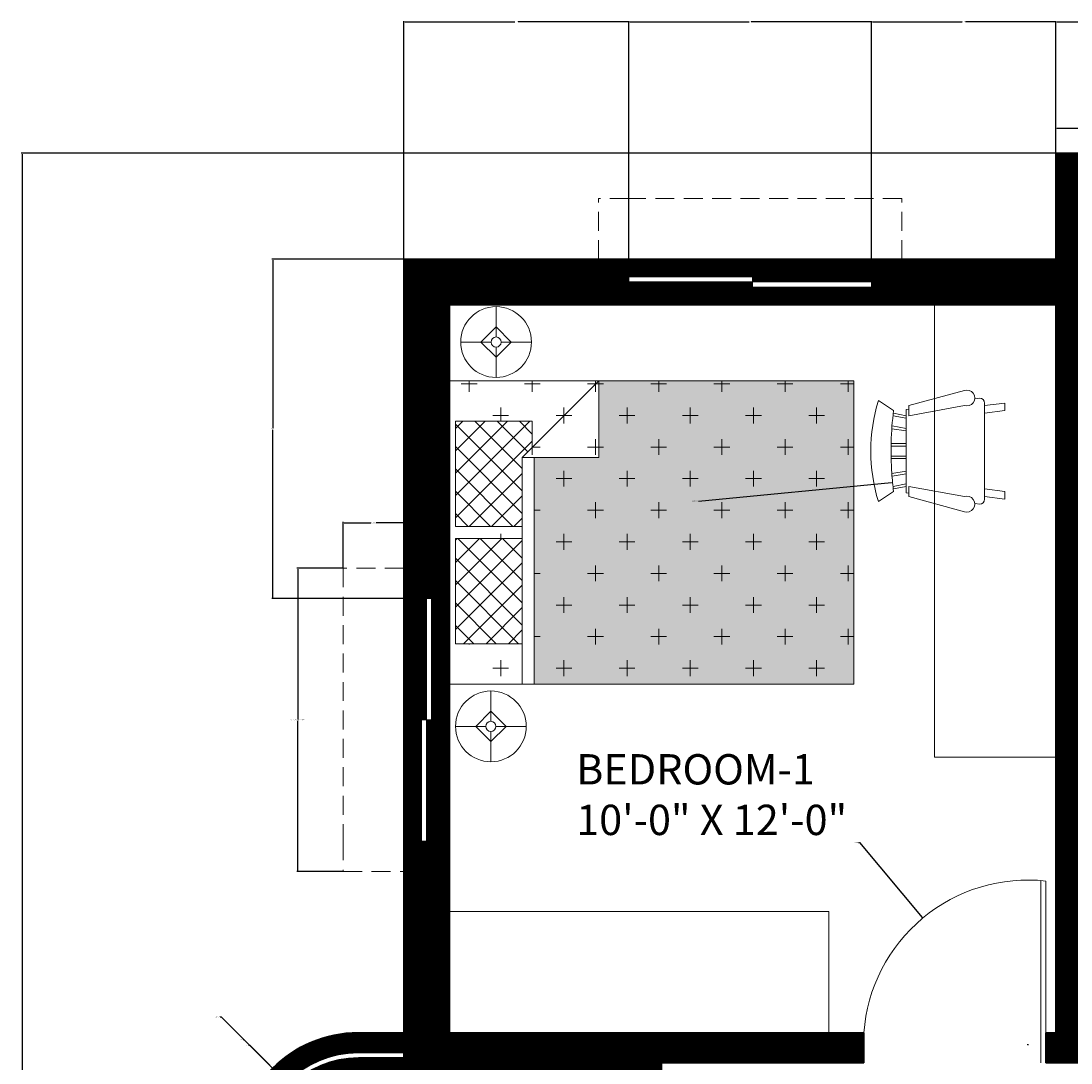
# Model space of a CAD drawing. Units: inches. Extents: x 557 to 1007, y 390 to 953.
# Tile 8 of 10: x 557 to 764, y 747 to 953. Entities that reach past the tile are written whole.
import ezdxf

# ---------------------------------------------------------------- set-up
doc = ezdxf.new("R2010")
doc.units = ezdxf.units.IN
doc.header["$LTSCALE"] = 5
doc.header["$MEASUREMENT"] = 0
doc.linetypes.add('HIDDEN', pattern=[0.375, 0.25, -0.125])
for name, color, linetype, lineweight in [('A-ANNO-DIMS', 2, 'Continuous', 18), ('A-AREA-IDEN', 7, 'Continuous', 18), ('A-DOOR', 3, 'Continuous', 18), ('A-FLOR-CASE', 8, 'Continuous', 18), ('A-FLOR-RAIL', 7, 'Continuous', 25), ('A-FURN', 8, 'Continuous', 18), ('A-FURN-PATT', 9, 'Continuous', 9), ('A-GLAZ', 4, 'Continuous', 18), ('A-GLAZ-OVHD', 8, 'HIDDEN', 13), ('A-WALL', 7, 'Continuous', 35), ('E-LITE', 2, 'Continuous', 13)]:
    doc.layers.add(name, color=color, linetype=linetype, lineweight=lineweight)
doc.layers.add('A-GLAZ-PATT', color=141, linetype='Continuous', lineweight=9, true_color=0xadddf7)
doc.layers.add('A-WALL-PATT', color=251, linetype='Continuous', lineweight=9, true_color=0x636466)
doc.styles.get("Standard").update_dxf_attribs({"font": 'arial.ttf'})
doc.dimstyles.get("Standard").update_dxf_attribs({"dimtxt": 0.18, "dimasz": 0.18, "dimexe": 0.18, "dimexo": 0.0625, "dimgap": 0.09, "dimtad": 0, "dimtih": 1, "dimtoh": 1, "dimdec": 4, "dimzin": 0, "dimdsep": 46, "dimtxsty": 'Standard', "dimcen": 0.09, "dimadec": 0, "dimazin": 0, "dimtfac": 1, "dimtdec": 4, "dimtofl": 0, "dimtmove": 0, "dimatfit": 3, "dimfxl": 1, "dimtolj": 1, "dimtzin": 0, "dimarcsym": 0})

# ---------------------------------------------------------------- blocks, each defined once
blk = doc.blocks.new('Chair - Rocking')
for p, q in [((-8, -4.5), (-10, -1.5)), ((8, -4.5), (10, -1.5)), ((-1.5, -4.05012), (-1.5, -7)), ((-1, -7), (-1, -4.05012)), ((1, -7), (1, -4.04655)), ((1.5, -4.05012), (1.5, -7)), ((-7.5, -4.5), (-7, -7)), ((-6.5, -7), (-7.02225, -4.43)), ((-4.5, -7), (-4.96674, -4.19951)), ((-4, -7), (-4.40532, -4.16272)), ((4, -7), (4.40187, -4.18694)), ((4.5, -7), (4.96761, -4.19437)), ((6.5, -7), (7, -4.4057)), ((7.5, -4.5), (7, -7)), ((-9, -7.5), (-12, -18.49999)), ((-7, -7.5), (-9, -7.5)), ((-9, -18.49999), (-7, -7.5)), ((-8.23428, -6.99939), (-8.3093, -7.47958)), ((-8.23041, -7), (8.23915, -7)), ((7, -7.5), (9, -7.5)), ((9, -18.49999), (7, -7.5)), ((8.31071, -7.48854), (8.23449, -7.00073)), ((9, -7.5), (12, -18.49999)), ((-10.36644, -20.64523), (-10.5, -21.49999)), ((10.5, -21.49999), (10.3575, -20.58798)), ((-9, -22.49999), (-9.5, -26.49999)), ((0, -22.49999), (-9.5, -22.49999)), ((-8, -26.49999), (-7.5, -22.49999)), ((0, -22.49999), (9.5, -22.49999)), ((8, -26.49999), (7.5, -22.49999)), ((9, -22.49999), (9.5, -26.49999)), ((-9.5, -26.49999), (-8, -26.49999)), ((9.5, -26.49999), (8, -26.49999))]:
    blk.add_line(p, q)
for centre, radius, start, end in [((0, -34.08333), 34.08333, 72.93847, 107.0615), ((0, -68.25004), 64.25, 93.92211, 97.15267), ((0, -68.25004), 64.25, 82.84733, 93.92211), ((-10.5, -18.99999), 1.58114, 161.5651, 18.43495), ((10.5, -18.99999), 1.58114, 161.5651, 18.43495), ((-9.5, -21.49999), 1, 180, 270), ((9.5, -21.49999), 1, 270, 0)]:
    blk.add_arc(centre, radius, start, end)
blk = doc.blocks.new('Lamp - Table')
for p, q in [((0, 7), (0, 1)), ((0, 3), (-3, 0)), ((3, 0), (0, 3)), ((-1, 0), (-7, 0)), ((-3, 0), (0, -3)), ((0, -3), (3, 0)), ((1, 0), (7, 0)), ((0, -1), (0, -7))]:
    blk.add_line(p, q)
for radius in [7, 1]:
    blk.add_circle((0, 0), radius)
blk = doc.blocks.new('BED-QUEEN-60x80-PLAN')
for p, q in [((0, 0), (0, 60)), ((0, 60), (80, 60)), ((29.6, 60), (14.4, 44.8)), ((29.6, 44.8), (29.6, 60)), ((80, 60), (80, 0)), ((1.2, 52), (16.4, 52)), ((1.2, 31.2), (1.2, 52)), ((16.4, 52), (16.4, 46.8)), ((14.4, 0), (14.4, 44.8)), ((14.4, 44.8), (29.6, 44.8)), ((16.8, 44.8), (16.8, 0)), ((14.4, 31.2), (1.2, 31.2)), ((1.2, 28.8), (14.4, 28.8)), ((1.2, 8), (1.2, 28.8)), ((14.4, 8), (1.2, 8)), ((80, 0), (0, 0))]:
    blk.add_line(p, q)
blk = doc.blocks.new('WIN-48-SLIDING')
for p, q in [((0, 9), (0, 0)), ((48, 9), (48, 0)), ((24, 5.5), (0, 5.5)), ((48, 4.5), (0, 4.5)), ((24, 5.5), (24, 3.5)), ((48, 3.5), (24, 3.5))]:
    blk.add_line(p, q)
blk = doc.blocks.new('WINDOW-SHADE-60')
at = {"ltscale": 3}
for p, q in [((12, 60), (0, 60)), ((0, 60), (0, 6)), ((12, 54), (12, 60)), ((0, 6), (0, 0)), ((0, 0), (12, 0))]:
    blk.add_line(p, q, dxfattribs=at)
blk = doc.blocks.new('*D35')
at = {"layer": 'A-ANNO-DIMS', "color": 0, "lineweight": -2, "ltscale": 5, "transparency": 16777216}
for p, q in [((620.34, 844.77), (611.23, 844.77)), ((611.41, 844.59), (611.41, 814.95)), ((611.41, 784.95), (611.41, 814.59)), ((620.34, 784.77), (611.23, 784.77))]:
    blk.add_line(p, q, dxfattribs=at)
at = {"layer": 'A-ANNO-DIMS', "color": 0, "ltscale": 5, "transparency": 16777216}
for points in [[(611.38, 844.59), (611.44, 844.59), (611.41, 844.77)], [(611.38, 784.95), (611.44, 784.95), (611.41, 784.77)]]:
    blk.add_solid(points, dxfattribs=at)
at = {"layer": 'Defpoints', "color": 0, "ltscale": 5, "transparency": 16777216}
for p in [(611.41, 844.77), (620.41, 844.77), (620.41, 784.77)]:
    blk.add_point(p, dxfattribs=at)
at = {"layer": 'A-ANNO-DIMS', "color": 0, "ltscale": 5, "transparency": 16777216, "insert": (611.41, 814.77), "char_height": 0.18, "attachment_point": 5}
blk.add_mtext('\\A1;WINDOW SHADE 60 TYP.', dxfattribs=at)
blk = doc.blocks.new('*D36')
at = {"layer": 'A-ANNO-DIMS', "color": 0, "lineweight": -2, "ltscale": 5, "transparency": 16777216}
for p, q in [((620.41, 844.83), (620.41, 853.95)), ((620.59, 853.77), (625.89, 853.77)), ((632.23, 853.77), (626.92, 853.77)), ((632.41, 844.83), (632.41, 853.95))]:
    blk.add_line(p, q, dxfattribs=at)
at = {"layer": 'A-ANNO-DIMS', "color": 0, "ltscale": 5, "transparency": 16777216}
for points in [[(620.59, 853.8), (620.59, 853.74), (620.41, 853.77)], [(632.23, 853.8), (632.23, 853.74), (632.41, 853.77)]]:
    blk.add_solid(points, dxfattribs=at)
at = {"layer": 'Defpoints', "color": 0, "ltscale": 5, "transparency": 16777216}
for p in [(632.41, 853.77), (620.41, 844.77), (632.41, 844.77)]:
    blk.add_point(p, dxfattribs=at)
at = {"layer": 'A-ANNO-DIMS', "color": 0, "ltscale": 5, "transparency": 16777216, "insert": (626.41, 853.77), "char_height": 0.18, "attachment_point": 5}
blk.add_mtext('\\A1;12 TYP.', dxfattribs=at)
blk = doc.blocks.new('*D46')
at = {"layer": 'A-ANNO-DIMS', "color": 0, "lineweight": -2, "ltscale": 5, "transparency": 16777216}
for p, q in [((761.34, 926.9), (556.69, 926.9)), ((556.87, 926.72), (556.87, 671.59)), ((556.87, 416.08), (556.87, 671.22)), ((773.34, 415.9), (556.69, 415.9))]:
    blk.add_line(p, q, dxfattribs=at)
at = {"layer": 'A-ANNO-DIMS', "color": 0, "ltscale": 5, "transparency": 16777216}
for points in [[(556.84, 926.72), (556.9, 926.72), (556.87, 926.9)], [(556.84, 416.08), (556.9, 416.08), (556.87, 415.9)]]:
    blk.add_solid(points, dxfattribs=at)
at = {"layer": 'Defpoints', "color": 0, "ltscale": 5, "transparency": 16777216}
for p in [(556.87, 926.9), (761.41, 926.9), (773.41, 415.9)]:
    blk.add_point(p, dxfattribs=at)
at = {"layer": 'A-ANNO-DIMS', "color": 0, "ltscale": 5, "transparency": 16777216, "insert": (556.87, 671.4), "char_height": 0.18, "attachment_point": 5}
blk.add_mtext('\\A1;511', dxfattribs=at)
blk = doc.blocks.new('*D47')
at = {"layer": 'A-ANNO-DIMS', "color": 0, "lineweight": -2, "ltscale": 5, "transparency": 16777216}
for p, q in [((632.41, 905.97), (632.41, 953.03)), ((632.59, 952.85), (654.33, 952.85)), ((676.73, 952.85), (654.99, 952.85)), ((676.91, 905.97), (676.91, 953.03))]:
    blk.add_line(p, q, dxfattribs=at)
at = {"layer": 'A-ANNO-DIMS', "color": 0, "ltscale": 5, "transparency": 16777216}
for points in [[(632.59, 952.88), (632.59, 952.82), (632.41, 952.85)], [(676.73, 952.88), (676.73, 952.82), (676.91, 952.85)]]:
    blk.add_solid(points, dxfattribs=at)
at = {"layer": 'Defpoints', "color": 0, "ltscale": 5, "transparency": 16777216}
for p in [(676.91, 952.85), (632.41, 905.9), (676.91, 905.9)]:
    blk.add_point(p, dxfattribs=at)
at = {"layer": 'A-ANNO-DIMS', "color": 0, "ltscale": 5, "transparency": 16777216, "insert": (654.66, 952.85), "char_height": 0.18, "attachment_point": 5}
blk.add_mtext('\\A1;44.5', dxfattribs=at)
blk = doc.blocks.new('*D48')
at = {"layer": 'A-ANNO-DIMS', "color": 0, "lineweight": -2, "ltscale": 5, "transparency": 16777216}
for p, q in [((676.91, 905.97), (676.91, 953.03)), ((677.09, 952.85), (700.69, 952.85)), ((724.73, 952.85), (701.13, 952.85)), ((724.91, 905.97), (724.91, 953.03))]:
    blk.add_line(p, q, dxfattribs=at)
at = {"layer": 'A-ANNO-DIMS', "color": 0, "ltscale": 5, "transparency": 16777216}
for points in [[(677.09, 952.88), (677.09, 952.82), (676.91, 952.85)], [(724.73, 952.88), (724.73, 952.82), (724.91, 952.85)]]:
    blk.add_solid(points, dxfattribs=at)
at = {"layer": 'Defpoints', "color": 0, "ltscale": 5, "transparency": 16777216}
for p in [(724.91, 952.85), (676.91, 905.9), (724.91, 905.9)]:
    blk.add_point(p, dxfattribs=at)
at = {"layer": 'A-ANNO-DIMS', "color": 0, "ltscale": 5, "transparency": 16777216, "insert": (700.91, 952.85), "char_height": 0.18, "attachment_point": 5}
blk.add_mtext('\\A1;48', dxfattribs=at)
blk = doc.blocks.new('*D49')
at = {"layer": 'A-ANNO-DIMS', "color": 0, "lineweight": -2, "ltscale": 5, "transparency": 16777216}
for p, q in [((724.91, 905.97), (724.91, 953.03)), ((725.09, 952.85), (742.83, 952.85)), ((761.23, 952.85), (743.48, 952.85)), ((761.41, 905.97), (761.41, 953.03))]:
    blk.add_line(p, q, dxfattribs=at)
at = {"layer": 'A-ANNO-DIMS', "color": 0, "ltscale": 5, "transparency": 16777216}
for points in [[(725.09, 952.88), (725.09, 952.82), (724.91, 952.85)], [(761.23, 952.88), (761.23, 952.82), (761.41, 952.85)]]:
    blk.add_solid(points, dxfattribs=at)
at = {"layer": 'Defpoints', "color": 0, "ltscale": 5, "transparency": 16777216}
for p in [(761.41, 952.85), (724.91, 905.9), (761.41, 905.9)]:
    blk.add_point(p, dxfattribs=at)
at = {"layer": 'A-ANNO-DIMS', "color": 0, "ltscale": 5, "transparency": 16777216, "insert": (743.16, 952.85), "char_height": 0.18, "attachment_point": 5}
blk.add_mtext('\\A1;36.5', dxfattribs=at)
blk = doc.blocks.new('*D50')
at = {"layer": 'A-ANNO-DIMS', "color": 0, "lineweight": -2, "ltscale": 5, "transparency": 16777216}
for p, q in [((761.41, 926.97), (761.41, 953.03)), ((761.59, 952.85), (803.19, 952.85)), ((845.23, 952.85), (803.62, 952.85)), ((845.41, 926.97), (845.41, 953.03))]:
    blk.add_line(p, q, dxfattribs=at)
at = {"layer": 'A-ANNO-DIMS', "color": 0, "ltscale": 5, "transparency": 16777216}
for points in [[(761.59, 952.88), (761.59, 952.82), (761.41, 952.85)], [(845.23, 952.88), (845.23, 952.82), (845.41, 952.85)]]:
    blk.add_solid(points, dxfattribs=at)
at = {"layer": 'Defpoints', "color": 0, "ltscale": 5, "transparency": 16777216}
for p in [(845.41, 952.85), (761.41, 926.9), (845.41, 926.9)]:
    blk.add_point(p, dxfattribs=at)
at = {"layer": 'A-ANNO-DIMS', "color": 0, "ltscale": 5, "transparency": 16777216, "insert": (803.41, 952.85), "char_height": 0.18, "attachment_point": 5}
blk.add_mtext('\\A1;84', dxfattribs=at)
blk = doc.blocks.new('*D67')
at = {"layer": 'A-ANNO-DIMS', "color": 0, "lineweight": -2, "ltscale": 5, "transparency": 16777216}
for p, q in [((632.34, 905.9), (606.28, 905.9)), ((606.46, 905.72), (606.46, 872.52)), ((606.46, 838.95), (606.46, 872.15)), ((632.34, 838.77), (606.28, 838.77))]:
    blk.add_line(p, q, dxfattribs=at)
at = {"layer": 'A-ANNO-DIMS', "color": 0, "ltscale": 5, "transparency": 16777216}
for points in [[(606.43, 905.72), (606.49, 905.72), (606.46, 905.9)], [(606.43, 838.95), (606.49, 838.95), (606.46, 838.77)]]:
    blk.add_solid(points, dxfattribs=at)
at = {"layer": 'Defpoints', "color": 0, "ltscale": 5, "transparency": 16777216}
for p in [(606.46, 905.9), (632.41, 905.9), (632.41, 838.77)]:
    blk.add_point(p, dxfattribs=at)
at = {"layer": 'A-ANNO-DIMS', "color": 0, "ltscale": 5, "transparency": 16777216, "insert": (606.46, 872.34), "char_height": 0.18, "attachment_point": 5}
blk.add_mtext('\\A1;67.14', dxfattribs=at)
blk = doc.blocks.new('*D76')
at = {"layer": 'A-ANNO-DIMS', "color": 0, "lineweight": -2, "ltscale": 5, "transparency": 16777216}
for p, q in [((761.41, 905.97), (761.41, 932.03)), ((761.59, 931.85), (784.34, 931.85)), ((807.88, 931.85), (785.13, 931.85)), ((808.06, 905.97), (808.06, 932.03))]:
    blk.add_line(p, q, dxfattribs=at)
at = {"layer": 'A-ANNO-DIMS', "color": 0, "ltscale": 5, "transparency": 16777216}
for points in [[(761.59, 931.88), (761.59, 931.82), (761.41, 931.85)], [(807.88, 931.88), (807.88, 931.82), (808.06, 931.85)]]:
    blk.add_solid(points, dxfattribs=at)
at = {"layer": 'Defpoints', "color": 0, "ltscale": 5, "transparency": 16777216}
for p in [(808.06, 931.85), (761.41, 905.9), (808.06, 905.9)]:
    blk.add_point(p, dxfattribs=at)
at = {"layer": 'A-ANNO-DIMS', "color": 0, "ltscale": 5, "transparency": 16777216, "insert": (784.73, 931.85), "char_height": 0.18, "attachment_point": 5}
blk.add_mtext('\\A1;46.66', dxfattribs=at)
blk = doc.blocks.new('*D101')
at = {"layer": 'A-ANNO-DIMS', "color": 0, "lineweight": -2, "ltscale": 5, "transparency": 16777216}
for p, q in [((596.07, 756.06), (596.25, 756.06)), ((596.25, 756.06), (606.31, 746)), ((623.32, 728.9), (623.5, 728.9)), ((623.41, 728.81), (623.41, 728.99))]:
    blk.add_line(p, q, dxfattribs=at)
at = {"layer": 'A-ANNO-DIMS', "color": 0, "ltscale": 5, "transparency": 16777216}
blk.add_solid([(606.33, 746.02), (606.29, 745.98), (606.43, 745.88)], dxfattribs=at)
at = {"layer": 'Defpoints', "color": 0, "ltscale": 5, "transparency": 16777216}
for p in [(606.43, 745.88), (623.41, 728.9)]:
    blk.add_point(p, dxfattribs=at)
at = {"layer": 'A-ANNO-DIMS', "color": 0, "ltscale": 5, "transparency": 16777216, "insert": (595.57, 756.06), "char_height": 0.18, "attachment_point": 5}
blk.add_mtext('\\A1;2X R24', dxfattribs=at)
blk = doc.blocks.new('*D102')
at = {"layer": 'A-ANNO-DIMS', "color": 0, "lineweight": -2, "ltscale": 5, "transparency": 16777216}
for p, q in [((600.6, 751.53), (600.78, 751.53)), ((600.78, 751.53), (609.14, 743.17)), ((623.32, 728.9), (623.5, 728.9)), ((623.41, 728.81), (623.41, 728.99))]:
    blk.add_line(p, q, dxfattribs=at)
at = {"layer": 'A-ANNO-DIMS', "color": 0, "ltscale": 5, "transparency": 16777216}
blk.add_solid([(609.16, 743.2), (609.11, 743.15), (609.26, 743.05)], dxfattribs=at)
at = {"layer": 'Defpoints', "color": 0, "ltscale": 5, "transparency": 16777216}
for p in [(609.26, 743.05), (623.41, 728.9)]:
    blk.add_point(p, dxfattribs=at)
at = {"layer": 'A-ANNO-DIMS', "color": 0, "ltscale": 5, "transparency": 16777216, "insert": (600.29, 751.53), "char_height": 0.18, "attachment_point": 5}
blk.add_mtext('\\A1;R20', dxfattribs=at)
blk = doc.blocks.new('*D103')
at = {"layer": 'A-ANNO-DIMS', "color": 0, "lineweight": -2, "ltscale": 5, "transparency": 16777216}
for p, q in [((601.73, 750.4), (601.91, 750.4)), ((601.91, 750.4), (609.84, 742.47)), ((623.32, 728.9), (623.5, 728.9)), ((623.41, 728.81), (623.41, 728.99))]:
    blk.add_line(p, q, dxfattribs=at)
at = {"layer": 'A-ANNO-DIMS', "color": 0, "ltscale": 5, "transparency": 16777216}
blk.add_solid([(609.86, 742.49), (609.82, 742.45), (609.97, 742.34)], dxfattribs=at)
at = {"layer": 'Defpoints', "color": 0, "ltscale": 5, "transparency": 16777216}
for p in [(609.97, 742.34), (623.41, 728.9)]:
    blk.add_point(p, dxfattribs=at)
at = {"layer": 'A-ANNO-DIMS', "color": 0, "ltscale": 5, "transparency": 16777216, "insert": (601.42, 750.4), "char_height": 0.18, "attachment_point": 5}
blk.add_mtext('\\A1;R19', dxfattribs=at)
blk = doc.blocks.new('*D106')
at = {"layer": 'A-ANNO-DIMS', "color": 0, "lineweight": -2, "ltscale": 5, "transparency": 16777216}
for p, q in [((722.35, 790.55), (722.53, 790.55)), ((722.53, 790.55), (734.91, 775.69)), ((755.77, 750.56), (755.95, 750.56)), ((755.86, 750.47), (755.86, 750.65))]:
    blk.add_line(p, q, dxfattribs=at)
at = {"layer": 'A-ANNO-DIMS', "color": 0, "ltscale": 5, "transparency": 16777216}
blk.add_solid([(734.94, 775.71), (734.89, 775.68), (735.03, 775.56)], dxfattribs=at)
at = {"layer": 'Defpoints', "color": 0, "ltscale": 5, "transparency": 16777216}
for p in [(735.03, 775.56), (755.86, 750.56)]:
    blk.add_point(p, dxfattribs=at)
at = {"layer": 'A-ANNO-DIMS', "color": 0, "ltscale": 5, "transparency": 16777216, "insert": (721.87, 790.55), "char_height": 0.18, "attachment_point": 5}
blk.add_mtext('\\A1;R32.54', dxfattribs=at)
blk = doc.blocks.new('*D112')
at = {"layer": 'A-ANNO-DIMS', "color": 0, "lineweight": -2, "ltscale": 5, "transparency": 16777216}
for p, q in [((792.94, 867.96), (793.12, 867.96)), ((793.03, 867.87), (793.03, 868.05)), ((690.71, 858.03), (728.9, 861.74))]:
    blk.add_line(p, q, dxfattribs=at)
at = {"layer": 'A-ANNO-DIMS', "color": 0, "ltscale": 5, "transparency": 16777216}
blk.add_solid([(728.9, 861.77), (728.91, 861.71), (729.08, 861.76)], dxfattribs=at)
at = {"layer": 'Defpoints', "color": 0, "ltscale": 5, "transparency": 16777216}
for p in [(793.03, 867.96), (729.08, 861.76)]:
    blk.add_point(p, dxfattribs=at)
at = {"layer": 'A-ANNO-DIMS', "color": 0, "ltscale": 5, "transparency": 16777216, "insert": (690.03, 858.03), "char_height": 0.18, "attachment_point": 5}
blk.add_mtext('\\A1;4X R64.25', dxfattribs=at)

msp = doc.modelspace()

# ---------------------------------------------------------------- hatches: boundary and pattern name
at = {"layer": 'A-FURN-PATT', "ltscale": 5}
h = msp.add_hatch(dxfattribs=at)
h.set_pattern_fill('GRAVEL', color=256, scale=25)
h.set_pattern_definition([(228.01279, (18, 25), (-200, -225), [3.3634, -332.9772]), (184.96974, (15.75, 22.5), (300, 25), [5.7717, -571.39812]), (132.51045, (10, 22), (250, -275), [4.0697, -402.9008]), (267.27369, (0.25, 15.75), (25, 500), [5.25595, -520.33895]), (292.83365, (0, 10.5), (-125, 300), [5.15387, -510.23433]), (357.27369, (2, 5.75), (-500, 25), [5.25595, -520.33895]), (37.69424, (7.25, 5.5), (-325, -250), [6.95072, -688.1212]), (72.25533, (12.75, 9.75), (175, 550), [6.5622, -649.65804]), (121.42957, (14.75, 16), (-200, 325), [5.27375, -522.10183]), (175.23636, (12, 20.5), (275, -25), [6.0208, -295.01906]), (222.39744, (6, 21), (-300, -275), [7.7862, -770.83438]), (138.81407, (25, 15.5), (-175, 150), [2.65752, -263.0961]), (171.46923, (23, 17.25), (325, -50), [5.05593, -500.5378]), (225, (18, 18), (-3e-15, -25), [3.53552, -31.8198]), (203.1986, (16.25, 21), (125, 50), [1.90395, -188.49038]), (291.8014, (14.5, 20.25), (-25, 75), [2.69257, -131.93655]), (30.96376, (15.5, 17.75), (75, 50), [4.37322, -141.40057]), (161.56505, (19.25, 20), (50, -25), [3.16228, -75.89467]), (16.38954, (0, 20.25), (250, 75), [4.43, -438.57113]), (70.34618, (4.25, 21.5), (-100, -275), [3.71652, -367.9352]), (293.1986, (19.25, 25), (-50, 125), [3.80788, -186.58645]), (343.61046, (20.75, 21.5), (-250, 75), [4.43, -438.57113]), (339.44395, (0, 4.75), (-125, 50), [4.272, -209.3281]), (294.77514, (4, 3.25), (-125, 275), [3.57945, -354.36608]), (66.8014, (19.5, 0), (50, 125), [3.80788, -186.58645]), (17.35402, (21, 3.5), (-325, -100), [4.19078, -414.8856]), (69.44395, (7.25, 0), (-50, -125), [2.136, -211.4641]), (101.30993, (18, 0), (-25, 100), [1.27475, -126.20074]), (165.96376, (17.75, 1.25), (75, -25), [5.15388, -97.92377]), (186.00901, (12.75, 2.5), (250, 25), [4.77625, -472.84808]), (303.69007, (15.5, 15.5), (-25, 50), [3.60555, -86.53323]), (353.15723, (17.5, 12.5), (425, -50), [6.29485, -623.18907]), (60.9454, (23.75, 11.75), (-100, -175), [2.5739, -254.81685]), (90, (25, 14), (-25, 25), [1.5, -23.5]), (120.25644, (12.25, 3.25), (100, -175), [3.4731, -343.838]), (48.01279, (10.5, 6.25), (200, 225), [6.7268, -329.6138]), (0, (15, 11.25), (25, 25), [6.5, -18.5]), (325.30485, (21.5, 11.25), (250, -175), [3.95285, -391.33186]), (254.0546, (24.75, 9), (-25, -100), [3.64005, -178.3627]), (207.64598, (23.75, 5.5), (-475, -250), [5.92662, -586.73685]), (175.42608, (18.5, 2.75), (-325, 25), [6.26997, -620.72684])])
h.paths.add_polyline_path([(615.2525, 688.5, 1), (640.7475, 688.5, 1)])
h.paths.add_polyline_path([(917.0544, 663.8414, 0.33333323), (915.2241, 665.6717), (882.2793, 665.6717, 0.33333323), (880.449, 663.8414), (880.449, 649.1992, 0.33333323), (882.2793, 647.369), (915.2241, 647.369, 0.33333323), (917.0544, 649.1992)])
h.paths.add_polyline_path([(828.0807, 699.7098), (756.0807, 699.7098), (756.0807, 663.7098), (828.0807, 663.7098)])
h.paths.add_polyline_path([(787.5651, 663.7098), (768.5964, 663.7098), (769.8463, 655.7098), (786.3151, 655.7098)])
h.paths.add_polyline_path([(815.5651, 663.7098), (796.5964, 663.7098), (797.8463, 655.7098), (814.3151, 655.7098)])
h.paths.add_polyline_path([(836.0807, 689.9442), (828.0807, 691.1942), (828.0807, 672.2255), (836.0807, 673.4755)])
h.paths.add_polyline_path([(756.0807, 691.1942), (748.0807, 689.9442), (748.0807, 673.4755), (756.0807, 672.2255)])
h.paths.add_polyline_path([(786.3151, 707.7098), (769.8463, 707.7098), (768.5964, 699.7098), (787.5651, 699.7098)])
h.paths.add_polyline_path([(814.3151, 707.7098), (797.8463, 707.7098), (796.5964, 699.7098), (815.5651, 699.7098)])
h.paths.add_polyline_path([(917.4362, 607.3575), (889.5896, 607.3575), (889.5896, 586.4726), (917.4362, 586.4726)])
h.paths.add_polyline_path([(721.4053, 881.8539), (671.0053, 881.8539), (671.0053, 866.6539), (658.2053, 866.6539), (658.2053, 821.8539), (721.4053, 821.8539)])
h.paths.add_polyline_path([(925.4053, 875.1046), (875.0053, 875.1046), (875.0053, 859.9046), (862.2053, 859.9046), (862.2053, 815.1046), (925.4053, 815.1046)])
h.paths.add_polyline_path([(721.4053, 558.9046), (671.0053, 558.9046), (671.0053, 543.7046), (658.2053, 543.7046), (658.2053, 498.9046), (721.4053, 498.9046)])
at = {"layer": 'A-FURN-PATT'}
h = msp.add_hatch(dxfattribs=at)
h.set_pattern_fill('CROSS', color=256, scale=25)
h.paths.add_polyline_path([(925.4053, 875.1046), (875.0053, 875.1046), (875.0053, 859.9046), (862.2053, 859.9046), (862.2053, 815.1046), (925.4053, 815.1046)])
h.paths.add_polyline_path([(721.4053, 881.8539), (671.0053, 881.8539), (671.0053, 866.6539), (658.2053, 866.6539), (658.2053, 821.8539), (721.4053, 821.8539)])
h.paths.add_polyline_path([(671.0053, 881.8539), (655.8053, 866.6539), (671.0053, 866.6539)], flags=17)
h.paths.add_polyline_path([(671.0053, 881.8539), (641.4053, 881.8539), (641.4053, 821.8539), (655.8053, 821.8539), (655.8053, 829.8539), (642.6053, 829.8539), (642.6053, 850.6539), (655.8053, 850.6539), (655.8053, 853.0539), (642.6053, 853.0539), (642.6053, 873.8539), (657.8053, 873.8539), (657.8053, 868.6539)])
h.paths.add_polyline_path([(875.0053, 875.1046), (859.8053, 859.9046), (875.0053, 859.9046)], flags=17)
h.paths.add_polyline_path([(875.0053, 875.1046), (845.4053, 875.1046), (845.4053, 815.1046), (859.8053, 815.1046), (859.8053, 823.1046), (846.6053, 823.1046), (846.6053, 843.9046), (859.8053, 843.9046), (859.8053, 846.3046), (846.6053, 846.3046), (846.6053, 867.1046), (861.8053, 867.1046), (861.8053, 861.9046)])
h.paths.add_polyline_path([(721.4053, 558.9046), (671.0053, 558.9046), (671.0053, 543.7046), (658.2053, 543.7046), (658.2053, 498.9046), (721.4053, 498.9046)])
h.paths.add_polyline_path([(671.0053, 558.9046), (641.4053, 558.9046), (641.4053, 498.9046), (655.8053, 498.9046), (655.8053, 506.9046), (642.6053, 506.9046), (642.6053, 527.7046), (655.8053, 527.7046), (655.8053, 530.1046), (642.6053, 530.1046), (642.6053, 550.9046), (657.8053, 550.9046), (657.8053, 545.7046)])
h.paths.add_polyline_path([(671.0053, 558.9046), (657.8053, 545.7046), (655.8053, 543.7046), (671.0053, 543.7046)], flags=17)
h.paths.add_polyline_path([(873.1461, 661.8773, 0.41421356), (868.1461, 666.8773, -0.12244426), (867.1516, 666.8773), (855.014, 666.8773), (855.014, 647.2429), (867.4581, 647.2429, -0.08537395), (868.1461, 647.2429, 0.41421356), (873.1461, 652.2429)])
h.paths.add_polyline_path([(917.0544, 663.8414, 0.33333323), (915.2241, 665.6717), (882.2793, 665.6717, 0.33333323), (880.449, 663.8414), (880.449, 649.1992, 0.33333323), (882.2793, 647.369), (915.2241, 647.369, 0.33333323), (917.0544, 649.1992)])
h.paths.add_polyline_path([(944.9465, 667.5202), (932.6561, 667.5202, -0.10407786), (931.8144, 667.5202, 0.41421356), (926.8144, 662.5202), (926.8144, 652.8858, 0.41421356), (931.8144, 647.8858, -0.05611627), (932.2647, 647.8858), (944.9465, 647.8858)])
h.paths.add_polyline_path([(928.8341, 635.542, 0.41421356), (923.8341, 640.542), (914.1997, 640.542, 0.41421356), (909.1997, 635.542), (909.1997, 622.4099), (923.8341, 622.4099, 0.41421356), (928.8341, 627.4099)])
h.paths.add_polyline_path([(909.1997, 635.542, 0.41421356), (904.1997, 640.542), (894.5653, 640.542, 0.41421356), (889.5653, 635.542), (889.5653, 622.4099), (909.1997, 622.4099)])
h.paths.add_polyline_path([(889.5653, 635.542, 0.41421356), (884.5653, 640.542), (874.9308, 640.542, 0.41421356), (869.9308, 635.542), (869.9308, 627.4099, 0.41421356), (874.9308, 622.4099), (889.5653, 622.4099)])
h = msp.add_hatch(dxfattribs=at)
h.set_pattern_fill('ANSI37', color=256, scale=25)
h.paths.add_polyline_path([(655.8053, 866.6539), (657.8053, 868.6539), (657.8053, 873.8539), (642.6053, 873.8539), (642.6053, 853.0539), (655.8053, 853.0539)])
h.paths.add_polyline_path([(655.8053, 850.6539), (642.6053, 850.6539), (642.6053, 829.8539), (655.8053, 829.8539)])
h.paths.add_polyline_path([(859.8053, 859.9046), (861.8053, 861.9046), (861.8053, 867.1046), (846.6053, 867.1046), (846.6053, 846.3046), (859.8053, 846.3046)])
h.paths.add_polyline_path([(859.8053, 843.9046), (846.6053, 843.9046), (846.6053, 823.1046), (859.8053, 823.1046)])
h.paths.add_polyline_path([(655.8053, 527.7046), (642.6053, 527.7046), (642.6053, 506.9046), (655.8053, 506.9046)])
h.paths.add_polyline_path([(657.8053, 545.7046), (657.8053, 550.9046), (642.6053, 550.9046), (642.6053, 530.1046), (655.8053, 530.1046), (655.8053, 543.7046)])
at = {"layer": 'A-GLAZ-PATT'}
h = msp.add_hatch(dxfattribs=at)
h.set_pattern_fill('ANSI31', color=256)
h.paths.add_polyline_path([(635.9053, 814.7688), (636.9053, 814.7688), (636.9053, 838.7688), (632.4053, 838.7688), (632.4053, 790.7688), (635.9053, 790.7688)])
h.paths.add_polyline_path([(641.4053, 838.7688), (637.9053, 838.7688), (637.9053, 814.7688), (636.9053, 814.7688), (636.9053, 790.7688), (641.4053, 790.7688)])
h.paths.add_polyline_path([(603.4053, 728.9046, -0.41421356), (623.4053, 748.9046), (632.4053, 748.9046), (632.4053, 752.9046), (623.4053, 752.9046, 0.41421356), (599.4053, 728.9046), (599.4053, 614.9046), (603.4053, 614.9046)])
h.paths.add_polyline_path([(632.4053, 743.9046), (632.4053, 747.9046), (623.4053, 747.9046, 0.41421356), (604.4053, 728.9046), (604.4053, 614.9046), (608.4053, 614.9046), (608.4053, 719.9046, -0.41421356)])
h.paths.add_polyline_path([(683.4053, 722.9046), (678.9053, 722.9046), (678.9053, 698.9046), (679.9053, 698.9046), (679.9053, 662.9046), (678.9053, 662.9046), (678.9053, 638.9046), (683.4053, 638.9046)])
h.paths.add_polyline_path([(678.9053, 698.9046), (677.9053, 698.9046), (677.9053, 722.9046), (674.4053, 722.9046), (674.4053, 638.9046), (677.9053, 638.9046), (677.9053, 662.9046), (678.9053, 662.9046)])
h.paths.add_polyline_path([(635.9053, 593.9046), (632.4053, 593.9046), (632.4053, 557.9046), (635.9053, 557.9046)])
h.paths.add_polyline_path([(641.4053, 593.9046), (637.9053, 593.9046), (637.9053, 557.9046), (641.4053, 557.9046)])
h.paths.add_polyline_path([(764.9579, 448.9046), (716.9579, 448.9046), (716.9579, 445.4046), (740.9579, 445.4046), (740.9579, 444.4046), (764.9579, 444.4046)])
h.paths.add_polyline_path([(764.9579, 443.4046), (740.9579, 443.4046), (740.9579, 444.4046), (716.9579, 444.4046), (716.9579, 439.9046), (764.9579, 439.9046)])
h.paths.add_polyline_path([(938.4053, 905.9046), (878.4053, 905.9046), (878.4053, 902.4046), (908.4053, 902.4046), (908.4053, 901.4046), (938.4053, 901.4046)])
h.paths.add_polyline_path([(938.4053, 900.4046), (908.4053, 900.4046), (908.4053, 901.4046), (878.4053, 901.4046), (878.4053, 896.9046), (938.4053, 896.9046)])
h.paths.add_polyline_path([(724.9087, 905.9046), (676.9087, 905.9046), (676.9087, 902.4046), (701.4053, 902.4046), (701.4053, 901.4046), (724.9087, 901.4046)])
h.paths.add_polyline_path([(724.9087, 900.4046), (701.4053, 900.4046), (701.4053, 901.4046), (676.9087, 901.4046), (676.9087, 896.9046), (724.9087, 896.9046)])
h.paths.add_polyline_path([(832.0625, 905.9046), (808.0625, 905.9046), (808.0625, 902.4046), (832.0625, 902.4046)])
h.paths.add_polyline_path([(832.0625, 900.4046), (808.0625, 900.4046), (808.0625, 896.9046), (832.0625, 896.9046)])
at = {"layer": 'A-WALL-PATT'}
h = msp.add_hatch(dxfattribs=at)
h.set_pattern_fill('ANSI31', color=256)
h.paths.add_polyline_path([(808.0625, 905.9046), (767.4053, 905.9046), (767.4053, 920.9046), (839.4053, 920.9046), (839.4053, 905.9046), (832.0625, 905.9046), (832.0625, 896.9046), (839.4053, 896.9046), (839.4053, 800.9046), (837.4053, 800.9046), (837.4053, 794.9046), (839.4053, 794.9046), (839.4053, 790.9046), (845.4053, 790.9046), (845.4053, 896.9046), (878.4053, 896.9046), (878.4053, 905.9046), (845.4053, 905.9046), (845.4053, 926.9046), (761.4053, 926.9046), (761.4053, 914.9046), (761.4053, 905.9046), (724.9087, 905.9046), (724.9087, 896.9046), (761.4053, 896.9046), (761.4053, 752.9046), (759.4053, 752.9046), (759.4053, 746.9046), (767.4053, 746.9046), (767.4053, 794.9046), (807.4053, 794.9046), (807.4053, 800.9046), (767.4053, 800.9046), (767.4053, 896.9046), (808.0625, 896.9046)])
h.paths.add_polyline_path([(676.9087, 905.9046), (632.4053, 905.9046), (632.4053, 838.7688), (641.4053, 838.7688), (641.4053, 881.8539), (641.4053, 896.9046), (676.9087, 896.9046)])
h.paths.add_polyline_path([(980.4053, 905.9046), (938.4053, 905.9046), (938.4053, 896.9046), (971.4053, 896.9046), (971.4053, 752.9046), (845.4053, 752.9046), (845.4053, 754.9046), (839.4053, 754.9046), (839.4053, 746.9046), (971.4053, 746.9046), (971.4053, 720.1788), (980.4053, 720.1788)])
h.paths.add_polyline_path([(723.4053, 752.9046), (641.4053, 752.9046), (641.4053, 790.7688), (632.4053, 790.7688), (632.4053, 743.9046), (674.4053, 743.9046), (674.4053, 722.9046), (683.4053, 722.9046), (683.4053, 746.9046), (723.4053, 746.9046)])
h.paths.add_polyline_path([(980.4053, 684.1788), (971.4053, 684.1788), (971.4053, 614.9046), (845.4053, 614.9046), (845.4053, 608.9046), (971.4053, 608.9046), (971.4053, 512.9046), (908.7697, 512.9046), (908.7697, 508.9046), (971.4053, 508.9046), (971.4053, 448.9046), (845.4053, 448.9046), (845.4053, 508.9046), (878.7697, 508.9046), (878.7697, 512.9046), (845.4053, 512.9046), (845.4053, 562.9046), (779.4053, 562.9046), (779.4053, 614.9046), (761.4053, 614.9046), (761.4053, 608.9046), (773.4053, 608.9046), (773.4053, 512.636), (779.4053, 512.636), (779.4053, 556.9046), (839.4053, 556.9046), (839.4053, 448.9046), (830.432, 448.9046), (830.432, 439.9046), (839.4053, 439.9046), (839.4053, 433.0506), (839.4053, 421.9046), (779.4053, 421.9046), (779.4053, 439.9046), (796.9656, 439.9046), (806.432, 439.9046), (806.432, 448.9046), (779.4053, 448.9046), (779.4053, 482.636), (773.4053, 482.636), (773.4053, 448.9046), (764.9579, 448.9046), (764.9579, 439.9046), (773.4053, 439.9046), (773.4053, 415.9046), (845.4053, 415.9046), (845.4053, 439.9046), (980.4053, 439.9046)])
h.paths.add_polyline_path([(716.9579, 448.9046), (641.4053, 448.9046), (641.4053, 557.9046), (632.4053, 557.9046), (632.4053, 439.9046), (716.9579, 439.9046)])
h.paths.add_polyline_path([(725.4053, 614.9046), (683.4053, 614.9046), (683.4053, 638.9046), (674.4053, 638.9046), (674.4053, 614.9046), (608.4053, 614.9046), (582.8236, 614.9046), (582.8236, 605.9046), (599.4053, 605.9046), (632.4053, 605.9046), (641.4053, 605.9046), (641.4053, 608.9046), (725.4053, 608.9046)])
h.paths.add_polyline_path([(641.4053, 605.9046), (632.4053, 605.9046), (632.4053, 593.9046), (641.4053, 593.9046)])

# ---------------------------------------------------------------- linework, layer by layer
at = {"layer": 'A-DOOR'}
for p, q in [((758.4053, 746.9046), (758.4053, 782.9046)), ((759.4053, 746.9046), (759.4053, 782.9046))]:
    msp.add_line(p, q, dxfattribs=at)
msp.add_arc((755.861, 750.5577), 32.5405, 83.74699, 175.864152, dxfattribs=at)
at = {"layer": 'A-FLOR-CASE'}
for p, q in [((737.4053, 896.9046), (737.4053, 807.4173)), ((737.4053, 807.4173), (761.4053, 807.4173)), ((641.4053, 776.9046), (716.4955, 776.9046)), ((716.4955, 752.9046), (716.4955, 776.9046))]:
    msp.add_line(p, q, dxfattribs=at)
at = {"layer": 'A-FLOR-RAIL'}
for points in [[(632.4053, 752.9046), (623.4053, 752.9046, 0.41421356), (599.4053, 728.9046), (599.4053, 614.9046)], [(632.4053, 748.9046), (623.4053, 748.9046, 0.41421356), (603.4053, 728.9046), (603.4053, 614.9046)], [(632.4053, 747.9046), (623.4053, 747.9046, 0.41421356), (604.4053, 728.9046), (604.4053, 614.9046)]]:
    msp.add_lwpolyline(points, format="xyb", dxfattribs=at)
at = {"layer": 'A-GLAZ'}
for p, q in [((676.9087, 896.9046), (676.9087, 905.9046)), ((724.9087, 896.9046), (724.9087, 905.9046)), ((701.4053, 902.4046), (676.9087, 902.4046)), ((701.4053, 900.4046), (701.4053, 902.4046)), ((724.9087, 901.4046), (676.9087, 901.4046)), ((724.9087, 900.4046), (701.4053, 900.4046)), ((637.9053, 814.7688), (635.9053, 814.7688))]:
    msp.add_line(p, q, dxfattribs=at)
at = {"layer": 'A-GLAZ-OVHD', "ltscale": 3}
for p, q in [((676.9087, 917.9046), (670.9087, 917.9046)), ((670.9087, 905.9046), (670.9087, 917.9046)), ((730.9087, 917.9046), (676.9087, 917.9046)), ((730.9087, 905.9046), (730.9087, 917.9046)), ((676.9087, 905.9046), (670.9087, 905.9046)), ((724.9087, 905.9046), (730.9087, 905.9046))]:
    msp.add_line(p, q, dxfattribs=at)
at = {"layer": 'A-WALL'}
for p, q in [((761.4053, 914.9046), (761.4053, 926.9046)), ((761.4053, 926.9046), (845.4053, 926.9046)), ((761.4053, 905.9046), (761.4053, 914.9046)), ((632.4053, 905.9046), (761.4053, 905.9046)), ((632.4053, 905.9046), (632.4053, 743.9046)), ((641.4053, 896.9046), (641.4053, 752.9046)), ((641.4053, 896.9046), (761.4053, 896.9046)), ((761.4053, 896.9046), (761.4053, 752.9046)), ((641.4053, 752.9046), (723.4053, 752.9046)), ((723.4053, 752.9046), (723.4053, 746.9046)), ((759.4053, 752.9046), (759.4053, 746.9046)), ((759.4053, 752.9046), (761.4053, 752.9046)), ((683.4053, 746.9046), (683.4053, 614.9046)), ((683.4053, 746.9046), (723.4053, 746.9046)), ((759.4053, 746.9046), (767.4053, 746.9046))]:
    msp.add_line(p, q, dxfattribs=at)

# ---------------------------------------------------------------- block references
at = {"layer": 'A-FURN'}
msp.add_blockref('BED-QUEEN-60x80-PLAN', (641.405, 821.8544), dxfattribs=at)
at = {"layer": 'A-FURN', "rotation": 90}
msp.add_blockref('Chair - Rocking', (724.7825, 867.9551), dxfattribs=at)
at = {"layer": 'A-GLAZ', "rotation": 90.00000000000006}
msp.add_blockref('WIN-48-SLIDING', (641.4048, 790.7689), dxfattribs=at)
at = {"layer": 'A-GLAZ-OVHD'}
msp.add_blockref('WINDOW-SHADE-60', (620.405, 784.769), dxfattribs=at)
at = {"layer": 'E-LITE', "rotation": 90}
for p in [(650.6505, 889.5262), (649.6207, 813.4981)]:
    msp.add_blockref('Lamp - Table', p, dxfattribs=at)

# ---------------------------------------------------------------- texts
at = {"layer": 'A-AREA-IDEN', "insert": (666.5, 808), "char_height": 6, "attachment_point": 1}
msp.add_mtext_dynamic_manual_height_columns('BEDROOM-1\\P10\'-0" X 12\'-0"', width=125, gutter_width=1, heights=[0], dxfattribs=at)

# ---------------------------------------------------------------- dimensions: what is measured, and where the dimension line sits
at = {"layer": 'A-ANNO-DIMS', "ltscale": 5}
for base, p1, p2, override, picture, middle in [((676.9087, 952.8546), (632.4053, 905.9046), (676.9087, 905.9046), {"dimdec": 1, "dimlfac": 1, "dimrnd": 0, "dimzin": 0, "dimdsep": 46, "dimlunit": 2}, '*D47', (654.657, 952.8546)), ((724.9087, 952.8546), (676.9087, 905.9046), (724.9087, 905.9046), {"dimdec": 0, "dimlfac": 1, "dimrnd": 0, "dimzin": 0, "dimdsep": 46, "dimlunit": 2}, '*D48', (700.9087, 952.8546)), ((761.4053, 952.8546), (724.9087, 905.9046), (761.4053, 905.9046), {"dimdec": 1, "dimlfac": 1, "dimrnd": 0, "dimzin": 0, "dimdsep": 46, "dimlunit": 2}, '*D49', (743.157, 952.8546)), ((845.4053, 952.8546), (761.4053, 926.9046), (845.4053, 926.9046), {"dimdec": 0, "dimlfac": 1, "dimrnd": 0, "dimzin": 0, "dimdsep": 46, "dimlunit": 2}, '*D50', (803.4053, 952.8546))]:
    dim = msp.add_linear_dim(base=base, p1=p1, p2=p2, dimstyle='Standard', override=override, dxfattribs=at)
    dim.commit()
    dim.dimension.update_dxf_attribs({"geometry": picture, "text_midpoint": middle})
for base, p1, p2, angle, override, picture, middle in [((808.0625, 931.8546), (761.4053, 905.9046), (808.0625, 905.9046), 0, {"dimdec": 2, "dimlfac": 1, "dimrnd": 0, "dimzin": 0, "dimdsep": 46, "dimlunit": 2}, '*D76', (784.7339, 931.8546)), ((556.8736, 926.9046), (773.4053, 415.9046), (761.4053, 926.9046), 90, {"dimdec": 0, "dimlfac": 1, "dimrnd": 0, "dimzin": 0, "dimdsep": 46, "dimlunit": 2}, '*D46', (556.8736, 671.4046)), ((606.4553, 905.9046), (632.4053, 838.7688), (632.4053, 905.9046), 90, {"dimdec": 2, "dimlfac": 1, "dimrnd": 0, "dimzin": 0, "dimdsep": 46, "dimlunit": 2}, '*D67', (606.4553, 872.3367))]:
    dim = msp.add_linear_dim(base=base, p1=p1, p2=p2, angle=angle, dimstyle='Standard', override=override, dxfattribs=at)
    dim.commit()
    dim.dimension.update_dxf_attribs({"geometry": picture, "text_midpoint": middle})
for center, mpoint, text, override, picture, middle in [((793.0326, 867.9551), (729.0824, 861.755), '4X <>', {"dimdec": 2, "dimlfac": 1, "dimrnd": 0, "dimzin": 0, "dimdsep": 46, "dimlunit": 2}, '*D112', (690.7124, 858.035)), ((623.4053, 728.9046), (606.4348, 745.8752), '2X <>', {"dimdec": 0, "dimlfac": 1, "dimrnd": 0, "dimzin": 0, "dimdsep": 46, "dimlunit": 2}, '*D101', (595.5729, 756.0576))]:
    dim = msp.add_radius_dim(center=center, mpoint=mpoint, text=text, dimstyle='Standard', override=override, dxfattribs=at)
    dim.commit()
    dim.dimension.update_dxf_attribs({"geometry": picture, "text_midpoint": middle, "dimtype": 164})
dim = msp.add_linear_dim(base=(632.4053, 853.7688), p1=(620.4053, 844.7688), p2=(632.4053, 844.7688), text='<> TYP.', dimstyle='Standard', override={"dimdec": 0, "dimlfac": 1, "dimrnd": 0, "dimzin": 0, "dimdsep": 46, "dimlunit": 2}, dxfattribs=at)
dim.commit()
dim.dimension.update_dxf_attribs({"geometry": '*D36', "text_midpoint": (626.4053, 853.7688)})
dim = msp.add_linear_dim(base=(611.4053, 844.7688), p1=(620.4053, 784.7688), p2=(620.4053, 844.7688), angle=90, text='WINDOW SHADE <> TYP.', dimstyle='Standard', override={"dimdec": 0, "dimlfac": 1, "dimrnd": 0, "dimzin": 0, "dimdsep": 46, "dimlunit": 2}, dxfattribs=at)
dim.commit()
dim.dimension.update_dxf_attribs({"geometry": '*D35', "text_midpoint": (611.4053, 814.7688)})
for center, mpoint, override, picture, middle in [((755.861, 750.5577), (735.029, 775.5559), {"dimdec": 2, "dimlfac": 1, "dimrnd": 0, "dimzin": 0, "dimdsep": 46, "dimlunit": 2}, '*D106', (721.8704, 790.5549)), ((623.4053, 728.9046), (609.2632, 743.0468), {"dimdec": 0, "dimlfac": 1, "dimrnd": 0, "dimzin": 0, "dimdsep": 46, "dimlunit": 2}, '*D102', (600.2932, 751.5321)), ((623.4053, 728.9046), (609.9703, 742.3397), {"dimdec": 0, "dimlfac": 1, "dimrnd": 0, "dimzin": 0, "dimdsep": 46, "dimlunit": 2}, '*D103', (601.4241, 750.4008))]:
    dim = msp.add_radius_dim(center=center, mpoint=mpoint, dimstyle='Standard', override=override, dxfattribs=at)
    dim.commit()
    dim.dimension.update_dxf_attribs({"geometry": picture, "text_midpoint": middle, "dimtype": 164})

doc.saveas('drawing.dxf')
